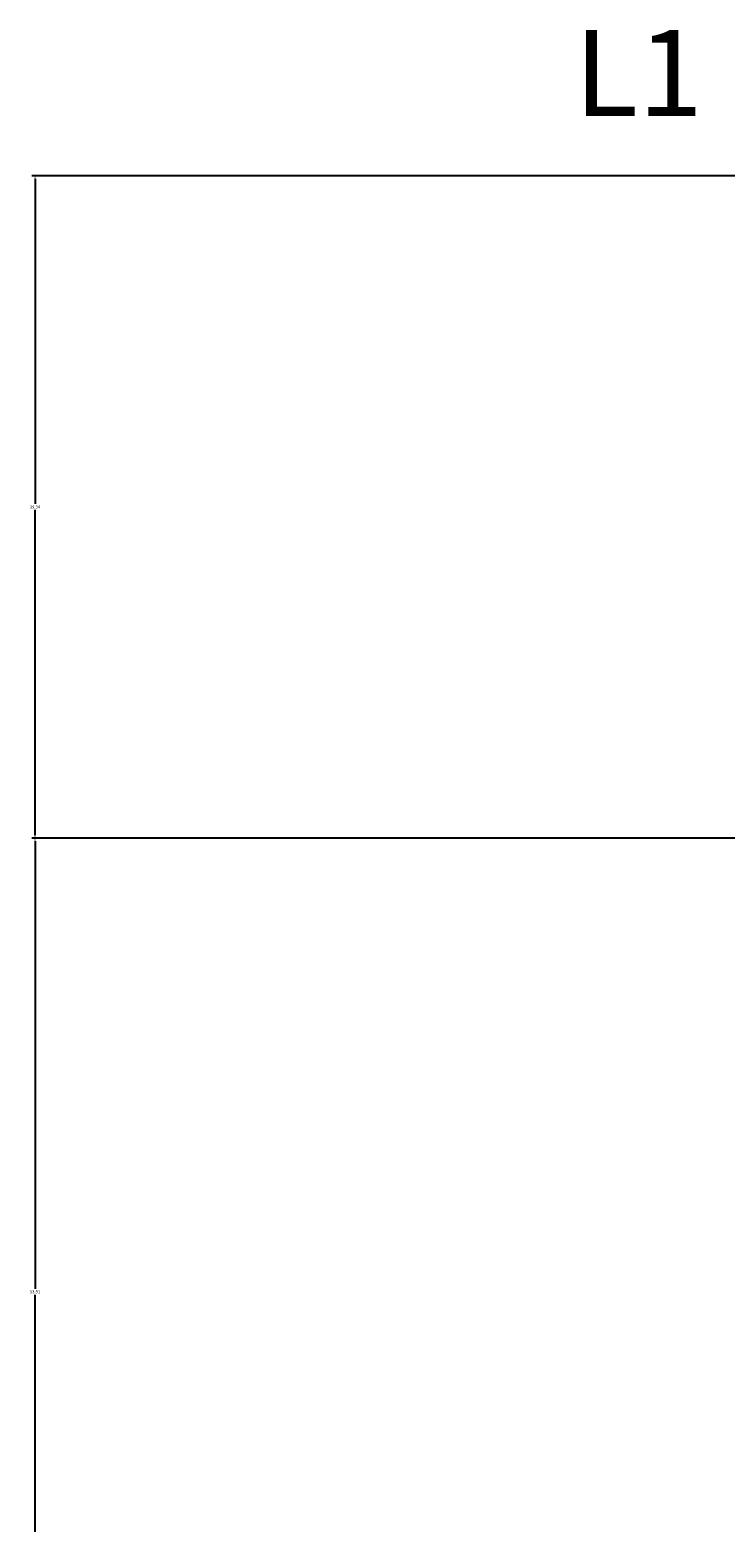
# Model space of a CAD drawing. Units: inches. Extents: x 738 to 1068, y 378 to 757.
# Tile 33 of 41: x 738 to 779, y 606 to 695. Entities that reach past the tile are written whole.
import ezdxf

# ---------------------------------------------------------------- set-up
doc = ezdxf.new("R2010")
doc.units = ezdxf.units.IN
doc.header["$MEASUREMENT"] = 0
doc.layers.add('A-ANNO-DIMS', color=2, linetype='Continuous', lineweight=18)
doc.layers.add('E-ANNO-TEXT', color=7, linetype='Continuous', lineweight=18)
doc.styles.get("Standard").update_dxf_attribs({"font": 'arial.ttf'})
doc.dimstyles.get("Standard").update_dxf_attribs({"dimtxt": 0.18, "dimasz": 0.18, "dimexe": 0.18, "dimexo": 0.0625, "dimgap": 0.09, "dimtad": 0, "dimtih": 1, "dimtoh": 1, "dimdec": 4, "dimzin": 0, "dimdsep": 46, "dimtxsty": 'Standard', "dimcen": 0.09, "dimadec": 0, "dimazin": 0, "dimtfac": 1, "dimtdec": 4, "dimtofl": 0, "dimtmove": 0, "dimatfit": 3, "dimfxl": 1, "dimtolj": 1, "dimtzin": 0, "dimarcsym": 0})

# ---------------------------------------------------------------- blocks, each defined once
blk = doc.blocks.new('*D23')
at = {"layer": 'A-ANNO-DIMS', "color": 0, "lineweight": -2, "transparency": 16777216}
for p, q in [((781.427, 646.985), (738.194, 646.985)), ((738.374, 646.805), (738.374, 620.214)), ((738.374, 593.26), (738.374, 619.85)), ((781.422, 593.08), (738.194, 593.08))]:
    blk.add_line(p, q, dxfattribs=at)
at = {"layer": 'A-ANNO-DIMS', "color": 0, "transparency": 16777216}
for points in [[(738.344, 646.805), (738.404, 646.805), (738.374, 646.985)], [(738.344, 593.26), (738.404, 593.26), (738.374, 593.08)]]:
    blk.add_solid(points, dxfattribs=at)
at = {"layer": 'Defpoints', "color": 0, "transparency": 16777216}
for p in [(738.374, 646.985), (781.49, 646.985), (781.485, 593.08)]:
    blk.add_point(p, dxfattribs=at)
at = {"layer": 'A-ANNO-DIMS', "color": 0, "transparency": 16777216, "insert": (738.374, 620.032), "char_height": 0.18, "attachment_point": 5}
blk.add_mtext('\\A1;53.91', dxfattribs=at)
blk = doc.blocks.new('*D24')
at = {"layer": 'A-ANNO-DIMS', "color": 0, "lineweight": -2, "transparency": 16777216}
for p, q in [((781.427, 686.329), (738.194, 686.329)), ((738.374, 686.149), (738.374, 666.839)), ((738.374, 647.165), (738.374, 666.475)), ((781.427, 646.985), (738.194, 646.985))]:
    blk.add_line(p, q, dxfattribs=at)
at = {"layer": 'A-ANNO-DIMS', "color": 0, "transparency": 16777216}
for points in [[(738.344, 686.149), (738.404, 686.149), (738.374, 686.329)], [(738.344, 647.165), (738.404, 647.165), (738.374, 646.985)]]:
    blk.add_solid(points, dxfattribs=at)
at = {"layer": 'Defpoints', "color": 0, "transparency": 16777216}
for p in [(738.374, 686.329), (781.49, 686.329), (781.49, 646.985)]:
    blk.add_point(p, dxfattribs=at)
at = {"layer": 'A-ANNO-DIMS', "color": 0, "transparency": 16777216, "insert": (738.374, 666.657), "char_height": 0.18, "attachment_point": 5}
blk.add_mtext('\\A1;39.34', dxfattribs=at)

msp = doc.modelspace()

# ---------------------------------------------------------------- texts
at = {"layer": 'E-ANNO-TEXT'}
msp.add_text('L1', height=5.11096, dxfattribs=at).set_placement((770.4075, 689.8867))

# ---------------------------------------------------------------- dimensions: what is measured, and where the dimension line sits
at = {"layer": 'A-ANNO-DIMS'}
for base, p1, p2, picture, middle in [((738.3736, 686.329), (781.4897, 646.9853), (781.4897, 686.329), '*D24', (738.3736, 666.6571)), ((738.3736, 646.9853), (781.4846, 593.0796), (781.4897, 646.9853), '*D23', (738.3736, 620.0325))]:
    dim = msp.add_linear_dim(base=base, p1=p1, p2=p2, angle=90, dimstyle='Standard', override={"dimdec": 2, "dimlfac": 1, "dimrnd": 0, "dimzin": 0, "dimdsep": 46, "dimlunit": 2}, dxfattribs=at)
    dim.commit()
    dim.dimension.update_dxf_attribs({"geometry": picture, "text_midpoint": middle})

doc.saveas('drawing.dxf')
